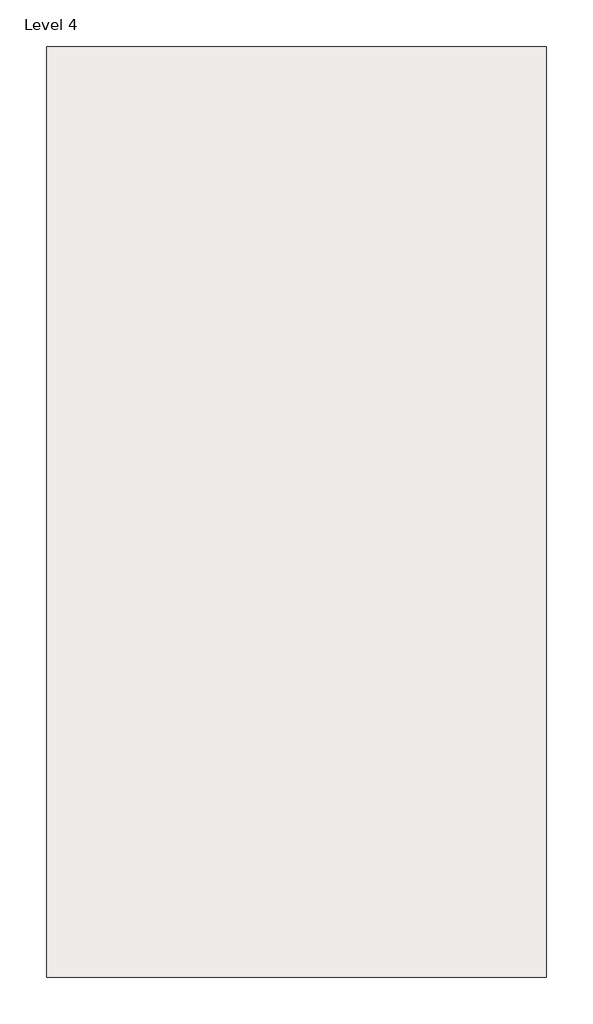
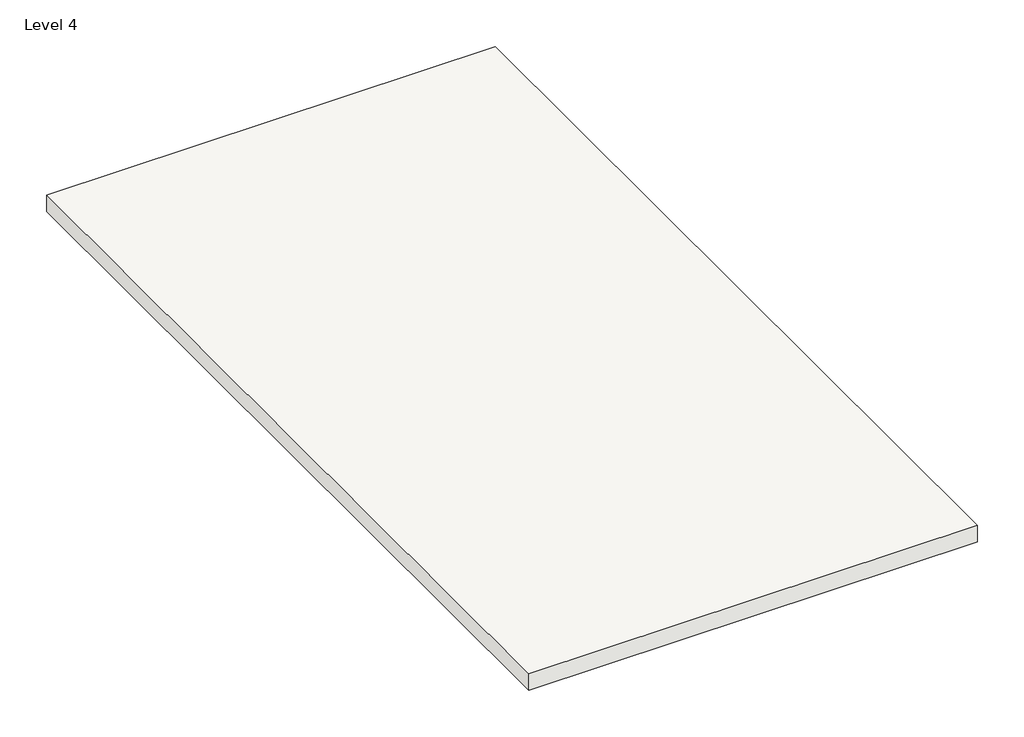
# One storey: 1 roof.
"""IFC4 building model written with IfcOpenShell, lengths in millimetres."""

from ifc_helpers import new_model, si_unit, frame, origin, place, context, project, spatial, polyline, outline, extrude, element, save

model = new_model("IFC4")

# Units and contexts
model_context = context("Model", 3, world=origin())
ifc_project = project(units=[si_unit("LENGTHUNIT", "METRE", prefix="MILLI")], contexts=[model_context])

# Site, building, storey
site = spatial("IfcSite", under=ifc_project)
building = spatial("IfcBuilding", under=site)
storey = spatial("IfcBuildingStorey", under=building, Name="Level 4", Elevation=6096.0)

# Roof
placement = place(None, origin())
element("IfcRoof", 1, ObjectType="SLAB", at=placement, inside=storey, context=model_context, shape_type="SweptSolid", body=[
    extrude(outline(polyline([(-4265.1844485, 2475.1269271), (-378.9844485, 2475.1269271), (-378.9844485, -4763.8730729), (-4265.1844485, -4763.8730729), (-4265.1844485, 2475.1269271)])), frame((0.0, 0.0, 6096.0), z_axis=(0.0, 0.0, 1.0), x_axis=(1.0, 0.0, 0.0)), (0.0, 0.0, 1.0), 152.4),
])

save(model, "model.ifc")

# Revit data of these elements
# Type "SLAB"
#   Assembly Code = "B1020"
#   Layers, outside or top first: 0' - 6" "SLAB" (function 1)
# Element 1 (IfcRoof, "SLAB")
#   built-in parameter 1001705 = 20.5 (stored number, unit not read)
#   built-in parameter 1001710 = 33615
#   Phase Created = New Construction
#   Materials on its faces: "SLAB"
# Materials
#   "SLAB": class "Generic", colour RGB 120 120 120, transparency 0, Cost = 0
